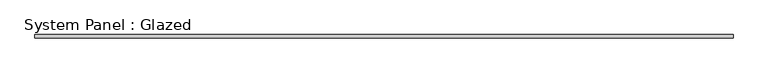
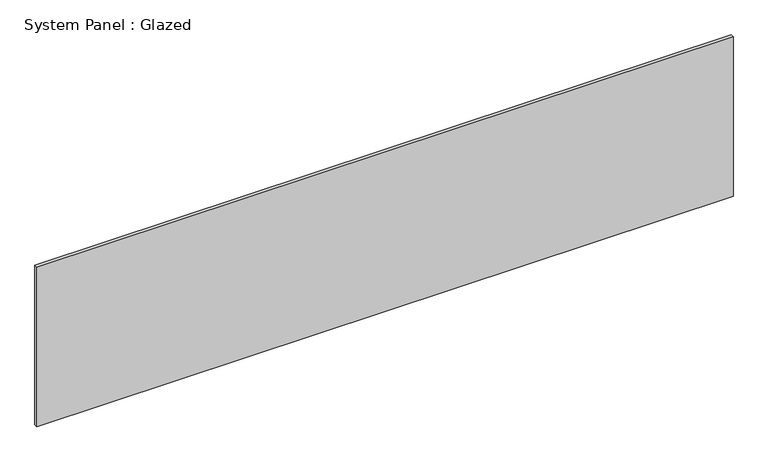
"""IFC4 building model written with IfcOpenShell, lengths in millimetres: plate geometry, System Panel : Glazed."""

from ifc_helpers import new_model, si_unit, origin, origin_with_axes, place, context, project, spatial, polyline, outline, extrude, source, transform, mapped, element, save


def system_panel_glazed_8ecd3908(model_context):
    return source(origin(), model_context, "Body", "SweptSolid", [
        extrude(outline(polyline([(2520.5006486, 19.05), (-2520.5006486, 19.05), (-2520.5006486, 44.45), (2520.5006486, 44.45), (2520.5006486, 19.05)])), origin_with_axes(), (0.0, 0.0, 1.0), 1219.2),
    ])


if __name__ == "__main__":
    model = new_model("IFC4")
    model_context = context("Model", 3, world=origin())
    ifc_project = project(units=[si_unit("LENGTHUNIT", "METRE", prefix="MILLI")], contexts=[model_context])
    site = spatial("IfcSite", under=ifc_project)
    building = spatial("IfcBuilding", under=site)
    placement = place(None, origin())
    system_panel_glazed_shape = system_panel_glazed_8ecd3908(model_context)
    element("IfcPlate", 1, ObjectType="System Panel : Glazed", at=placement, inside=building, context=model_context, shape_type="MappedRepresentation", body=[
        mapped(system_panel_glazed_shape, transform((0.0, 0.0, 0.0), x_axis=(1.0, 0.0, 0.0), y_axis=(0.0, 1.0, 0.0), z_axis=(0.0, 0.0, 1.0))),
    ])
    save(model, "model.ifc")

# Revit data of these elements
# Type "System Panel : Glazed"
#   Construction Type Id = "GSP4R"
#   Analytic Construction = "1/8 in Pilkington single glazing"
#   Visual Light Transmittance = 0.9
#   Solar Heat Gain Coefficient = 0.86
#   Heat Transfer Coefficient (U) = 1.18115 BTU/(h·ft²·°F)
# Element 1 (IfcPlate, "System Panel : Glazed")
#   Materials on its faces: "Glass"
# Materials
#   "Glass": class "Glass", colour RGB 0 128 192, transparency 0.75, Description = "Soda Lime Glass", Cost = 0
